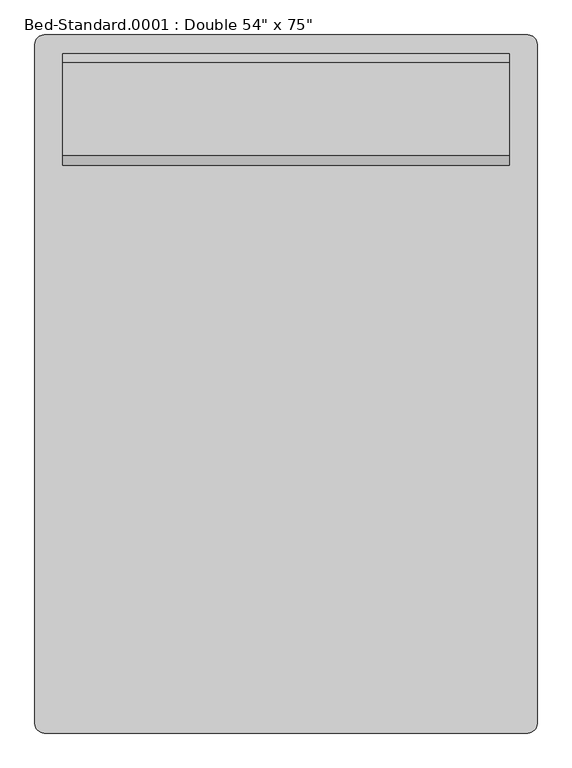
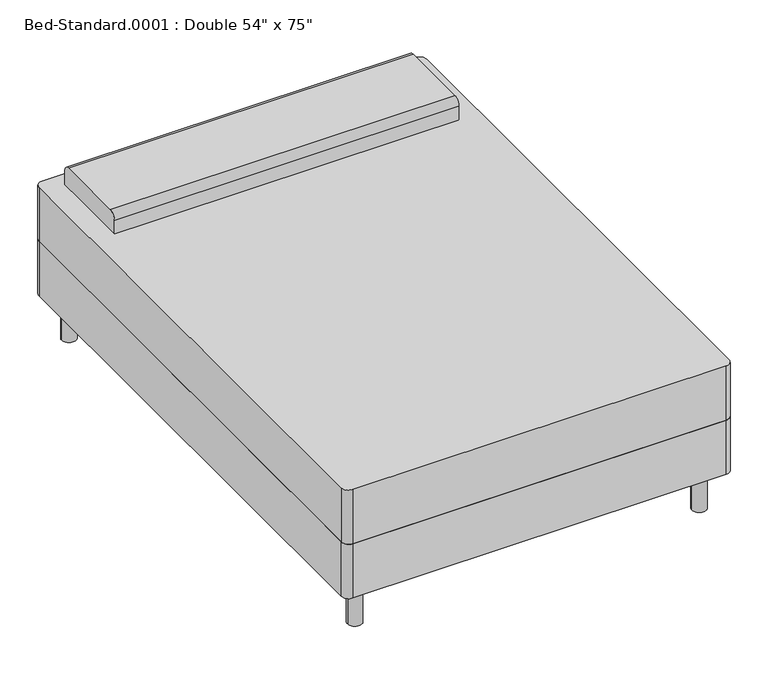
"""IFC4 building model written with IfcOpenShell, lengths in millimetres: furniture geometry."""

from ifc_helpers import new_model, si_unit, point, frame, frame_2d, origin, origin_with_axes, place, context, project, spatial, polyline, circle_curve, trimmed, segment, composite_curve, outline, extrude, source, transform, mapped, element, save


def furniture_0253826f(model_context):
    return source(origin(), model_context, "Body", "SweptSolid", [
        extrude(outline(composite_curve([segment(polyline([(-414.3114754, -972.695082), (-414.3114754, 881.504918)]), True, "CONTINUOUS"), segment(trimmed(circle_curve(frame_2d((-388.9114754, 881.504918)), 25.4), [point((-414.3114754, 881.504918))], [point((-388.9114754, 906.904918))], False, "CARTESIAN"), True, "CONTINUOUS"), segment(polyline([(-388.9114754, 906.904918), (931.8885246, 906.904918)]), True, "CONTINUOUS"), segment(trimmed(circle_curve(frame_2d((931.8885246, 881.504918)), 25.4), [point((931.8885246, 906.904918))], [point((957.2885246, 881.504918))], False, "CARTESIAN"), True, "CONTINUOUS"), segment(polyline([(957.2885246, 881.504918), (957.2885246, -972.695082)]), True, "CONTINUOUS"), segment(trimmed(circle_curve(frame_2d((931.8885246, -972.695082)), 25.4), [point((957.2885246, -972.695082))], [point((931.8885246, -998.095082))], False, "CARTESIAN"), True, "CONTINUOUS"), segment(polyline([(931.8885246, -998.095082), (-388.9114754, -998.095082)]), True, "CONTINUOUS"), segment(trimmed(circle_curve(frame_2d((-388.9114754, -972.695082)), 25.4), [point((-388.9114754, -998.095082))], [point((-414.3114754, -972.695082))], False, "CARTESIAN"), True, "CONTINUOUS")], self_intersect=False)), frame((0.0, 0.0, 152.4), z_axis=(0.0, 0.0, 1.0), x_axis=(1.0, 0.0, 0.0)), (0.0, 0.0, 1.0), 203.2),
        extrude(outline(composite_curve([segment(polyline([(551.304918, 558.8), (551.304918, 609.6)]), True, "CONTINUOUS"), segment(trimmed(circle_curve(frame_2d((576.704918, 609.6)), 25.4), [point((551.304918, 609.6))], [point((576.704918, 635.0))], False, "CARTESIAN"), True, "CONTINUOUS"), segment(polyline([(576.704918, 635.0), (830.704918, 635.0)]), True, "CONTINUOUS"), segment(trimmed(circle_curve(frame_2d((830.704918, 609.6)), 25.4), [point((830.704918, 635.0))], [point((856.104918, 609.6))], False, "CARTESIAN"), True, "CONTINUOUS"), segment(polyline([(856.104918, 609.6), (856.104918, 558.8), (551.304918, 558.8)]), True, "CONTINUOUS")], self_intersect=False)), frame((-338.1114754, 0.0, 0.0), z_axis=(1.0, 0.0, 0.0), x_axis=(0.0, 1.0, 0.0)), (0.0, 0.0, 1.0), 1219.2),
        extrude(outline(composite_curve([segment(trimmed(circle_curve(frame_2d((-338.1114754, 830.704918)), 25.4), [point((-363.5114754, 830.704918))], [point((-312.7114754, 830.704918))], False, "CARTESIAN"), True, "CONTINUOUS"), segment(trimmed(circle_curve(frame_2d((-338.1114754, 830.704918)), 25.4), [point((-312.7114754, 830.704918))], [point((-363.5114754, 830.704918))], False, "CARTESIAN"), True, "CONTINUOUS")], self_intersect=False)), origin_with_axes(), (0.0, 0.0, 1.0), 152.4),
        extrude(outline(composite_curve([segment(trimmed(circle_curve(frame_2d((881.0885246, 830.704918)), 25.4), [point((855.6885246, 830.704918))], [point((906.4885246, 830.704918))], False, "CARTESIAN"), True, "CONTINUOUS"), segment(trimmed(circle_curve(frame_2d((881.0885246, 830.704918)), 25.4), [point((906.4885246, 830.704918))], [point((855.6885246, 830.704918))], False, "CARTESIAN"), True, "CONTINUOUS")], self_intersect=False)), origin_with_axes(), (0.0, 0.0, 1.0), 152.4),
        extrude(outline(composite_curve([segment(trimmed(circle_curve(frame_2d((881.0885246, -921.895082)), 25.4), [point((855.6885246, -921.895082))], [point((906.4885246, -921.895082))], False, "CARTESIAN"), True, "CONTINUOUS"), segment(trimmed(circle_curve(frame_2d((881.0885246, -921.895082)), 25.4), [point((906.4885246, -921.895082))], [point((855.6885246, -921.895082))], False, "CARTESIAN"), True, "CONTINUOUS")], self_intersect=False)), origin_with_axes(), (0.0, 0.0, 1.0), 152.4),
        extrude(outline(composite_curve([segment(trimmed(circle_curve(frame_2d((-338.1114754, -921.895082)), 25.4), [point((-363.5114754, -921.895082))], [point((-312.7114754, -921.895082))], False, "CARTESIAN"), True, "CONTINUOUS"), segment(trimmed(circle_curve(frame_2d((-338.1114754, -921.895082)), 25.4), [point((-312.7114754, -921.895082))], [point((-363.5114754, -921.895082))], False, "CARTESIAN"), True, "CONTINUOUS")], self_intersect=False)), origin_with_axes(), (0.0, 0.0, 1.0), 152.4),
        extrude(outline(composite_curve([segment(polyline([(-388.9114754, 906.904918), (931.8885246, 906.904918)]), True, "CONTINUOUS"), segment(trimmed(circle_curve(frame_2d((931.8885246, 881.504918)), 25.4), [point((931.8885246, 906.904918))], [point((957.2885246, 881.504918))], False, "CARTESIAN"), True, "CONTINUOUS"), segment(polyline([(957.2885246, 881.504918), (957.2885246, -972.695082)]), True, "CONTINUOUS"), segment(trimmed(circle_curve(frame_2d((931.8885246, -972.695082)), 25.4), [point((957.2885246, -972.695082))], [point((931.8885246, -998.095082))], False, "CARTESIAN"), True, "CONTINUOUS"), segment(polyline([(931.8885246, -998.095082), (-388.9114754, -998.095082)]), True, "CONTINUOUS"), segment(trimmed(circle_curve(frame_2d((-388.9114754, -972.695082)), 25.4), [point((-388.9114754, -998.095082))], [point((-414.3114754, -972.695082))], False, "CARTESIAN"), True, "CONTINUOUS"), segment(polyline([(-414.3114754, -972.695082), (-414.3114754, 881.504918)]), True, "CONTINUOUS"), segment(trimmed(circle_curve(frame_2d((-388.9114754, 881.504918)), 25.4), [point((-414.3114754, 881.504918))], [point((-388.9114754, 906.904918))], False, "CARTESIAN"), True, "CONTINUOUS")], self_intersect=False)), frame((0.0, 0.0, 355.6), z_axis=(0.0, 0.0, 1.0), x_axis=(1.0, 0.0, 0.0)), (0.0, 0.0, 1.0), 203.2),
    ])


if __name__ == "__main__":
    model = new_model("IFC4")
    model_context = context("Model", 3, world=origin())
    ifc_project = project(units=[si_unit("LENGTHUNIT", "METRE", prefix="MILLI")], contexts=[model_context])
    site = spatial("IfcSite", under=ifc_project)
    building = spatial("IfcBuilding", under=site)
    placement = place(None, origin())
    furniture_shape = furniture_0253826f(model_context)
    element("IfcFurniture", 1, ObjectType="Bed-Standard.0001 : Double 54\" x 75\"", at=placement, inside=building, context=model_context, shape_type="MappedRepresentation", body=[
        mapped(furniture_shape, transform((0.0, 0.0, 0.0), x_axis=(1.0, 0.0, 0.0), y_axis=(0.0, 1.0, 0.0), z_axis=(0.0, 0.0, 1.0))),
    ])
    save(model, "model.ifc")

# Revit data of these elements
# Type "Bed-Standard.0001 : Double 54\" x 75\""
#   Assembly Code = "E2020200"
#   Length = 6' - 3"
#   Width = 4' - 6"
#   Leg Material = Steel, Chrome Plated
#   Mattress Material = Sash
#   Default Elevation = 0
# Element 1 (IfcFurniture, "Bed-Standard.0001 : Double 54\" x 75\"")
#   Materials on its faces: "Linen, White", "Steel, Chrome Plated"
# Materials
#   "Steel, Chrome Plated": class "Metal", colour RGB 17 17 17, transparency 0, Description = "Chromiuim plated steel", Cost = 0
#   "Sash": class "Wood", colour RGB 224 178 126, transparency 0
#   "Linen, White": class "Textile", colour RGB 247 247 239, transparency 0, Description = "Linen, white", Cost = 0
